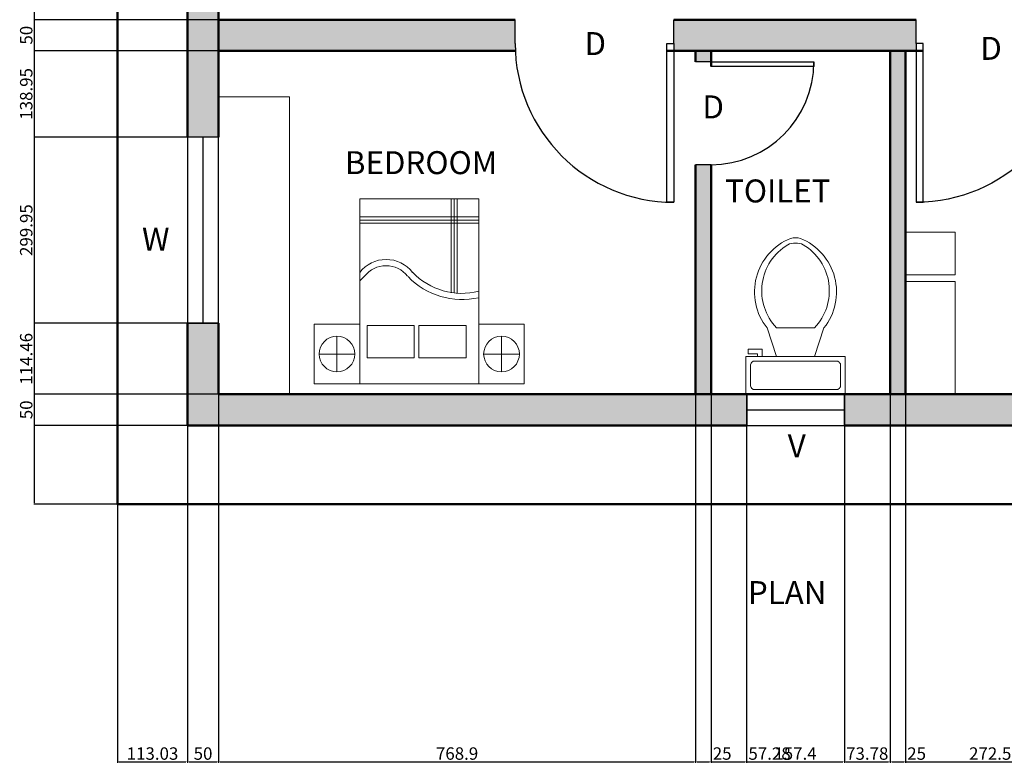
# Model space of a CAD drawing. Units: millimetres. Extents: x 1898 to 8115, y 727 to 4291.
# Tile 3 of 7: x 5191 to 6778, y 1079 to 2277. Entities that reach past the tile are written whole.
import ezdxf

# ---------------------------------------------------------------- set-up
doc = ezdxf.new("R2010")
doc.units = ezdxf.units.MM
for name, color, linetype, lineweight in [('A-ANNO-DIMS', 2, 'Continuous', 18), ('A-ANNO-TEXT', 7, 'Continuous', 25), ('A-AREA-IDEN', 3, 'Continuous', 25), ('A-DOOR', 3, 'Continuous', 25), ('A-FLOR-FIXT', 9, 'Continuous', 18), ('A-FURN', 8, 'Continuous', 18), ('A-GLAZ', 4, 'Continuous', 25), ('A-WALL', 7, 'Continuous', 50), ('A-WALL-PATT', 8, 'Continuous', 13)]:
    doc.layers.add(name, color=color, linetype=linetype, lineweight=lineweight)
doc.styles.get("Standard").update_dxf_attribs({"font": 'arial.ttf'})
doc.dimstyles.new('ISO-25', dxfattribs={"dimtxt": 20, "dimasz": 2.5, "dimexe": 1.25, "dimexo": 0.625, "dimtad": 1, "dimtxsty": 'Standard', "dimcen": 2.5, "dimadec": 0, "dimazin": 0, "dimtfac": 1, "dimtmove": 0, "dimatfit": 3, "dimfxl": 1, "dimarcsym": 0})

# ---------------------------------------------------------------- blocks, each defined once
blk = doc.blocks.new('*U43')
for p, q in [((0, 0), (0, -6)), ((40, 0), (40, -6))]:
    blk.add_line(p, q)
blk.add_lwpolyline([(0, 0), (0, 40), (1.75, 40), (1.75, 0)], close=True)
blk.add_arc((0, 0), 40, 0, 90)
blk = doc.blocks.new('*U45')
for p, q in [((9.5, -6), (9.5, -2)), ((-8, -8.5), (-8, -8)), ((-7, -8), (-7, -9.5)), ((-4, -8), (-6, -14)), ((4, -8), (6, -14)), ((-10, -8.5), (-8, -8.5)), ((-10, -9.5), (-10, -8.5)), ((-7, -9.5), (-10, -9.5)), ((4, -14), (-4, -14))]:
    blk.add_line(p, q)
blk.add_lwpolyline([(10.5, -8), (10.5, 0), (-10.5, 0), (-10.5, -8)], close=True)
for points in [[(-9.5, -2), (-9.5, -6)], [(8.5, -1), (-8.5, -1)], [(-8.5, -7), (8.5, -7)]]:
    blk.add_lwpolyline(points)
for centre, radius, start, end in [((-8.62, -1.88), 0.884, 81.8699, 188.1301), ((8.62, -1.88), 0.884, 351.8699, 98.1301), ((-8.62, -6.12), 0.884, 171.8699, 278.1301), ((8.62, -6.12), 0.884, 261.8699, 8.1301), ((3.52, -21.58), 12.17, 141.4691, 247.9714), ((4.2, -21.82), 11.33, 136.3677, 238.9468), ((-3.52, -21.58), 12.17, 292.0284, 38.5307), ((-4.2, -21.82), 11.33, 301.053, 43.6321), ((0, -27.88), 4, 245.7318, 294.2682), ((0, -29), 4, 254.8605, 285.1395)]:
    blk.add_arc(centre, radius, start, end)
blk = doc.blocks.new('BED-DOUBLE-SET')
for p, q in [((5578.8, 3262.9), (5578.8, 3320.5)), ((5550, 3291.7), (5607.6, 3291.7)), ((5704.8, 3246.7), (5696.6, 3255)), ((5789.5, 3063.1), (5789.5, 3255)), ((5794.5, 3063.1), (5794.5, 3255)), ((5799.5, 3063.1), (5799.5, 3255)), ((5677.2, 3107.9), (5828.6, 3107.9)), ((5677.2, 3102.9), (5828.6, 3102.9)), ((5677.2, 3097.9), (5828.6, 3097.9)), ((5578.8, 2997.7), (5578.8, 3055.3)), ((5550, 3026.5), (5607.6, 3026.5))]:
    blk.add_line(p, q)
for points in [[(5530.8, 3255), (5626.9, 3255), (5626.9, 3328.4), (5530.8, 3328.4)], [(5530.8, 3255), (5828.6, 3255), (5828.6, 3063.1), (5530.8, 3063.1)], [(5572.7, 3167.2), (5624.7, 3167.2), (5624.7, 3243.2), (5572.7, 3243.2)], [(5572.7, 3083.7), (5624.7, 3083.7), (5624.7, 3159.7), (5572.7, 3159.7)], [(5530.8, 2989.8), (5626.9, 2989.8), (5626.9, 3063.1), (5530.8, 3063.1)]]:
    blk.add_lwpolyline(points, close=True)
for centre in [(5578.8, 3291.7), (5578.8, 3026.5)]:
    blk.add_circle(centre, 28.8)
for centre, radius, start, end in [((5677.1, 3212.5), 54, 307.9745, 52.0255), ((5677.1, 3212.5), 44, 307.9745, 52.0255), ((5787.6, 3090), 121.1, 134.0052, 192.8109), ((5787.6, 3090), 111.1, 134.0052, 193.986)]:
    blk.add_arc(centre, radius, start, end)
blk = doc.blocks.new('*D59')
at = {"layer": 'A-ANNO-DIMS', "color": 0, "lineweight": -2, "transparency": 16777216}
for p, q in [((5347.9, 3559.7), (5213.8, 3559.7)), ((5215.1, 1499), (5215.1, 3557.2)), ((5347.9, 1496.5), (5213.8, 1496.5))]:
    blk.add_line(p, q, dxfattribs=at)
at = {"layer": 'A-ANNO-DIMS', "color": 0, "transparency": 16777216}
for points in [[(5214.6, 3557.2), (5215.5, 3557.2), (5215.1, 3559.7)], [(5214.6, 1499), (5215.5, 1499), (5215.1, 1496.5)]]:
    blk.add_solid(points, dxfattribs=at)
at = {"layer": 'Defpoints', "color": 0, "transparency": 16777216}
for p in [(5215.1, 3559.7), (5348.6, 3559.7), (5348.6, 1496.5)]:
    blk.add_point(p, dxfattribs=at)
at = {"layer": 'A-ANNO-DIMS', "color": 0, "transparency": 16777216, "insert": (5204.2, 2528.1), "char_height": 20, "attachment_point": 5, "rotation": 90}
blk.add_mtext('2063', dxfattribs=at)
blk = doc.blocks.new('*D60')
at = {"layer": 'A-ANNO-DIMS', "color": 0, "lineweight": -2, "transparency": 16777216}
for p, q in [((5461, 3440.7), (5213.8, 3440.7)), ((5215.1, 1626.1), (5215.1, 3438.2)), ((5461, 1623.6), (5213.8, 1623.6))]:
    blk.add_line(p, q, dxfattribs=at)
at = {"layer": 'A-ANNO-DIMS', "color": 0, "transparency": 16777216}
for points in [[(5214.6, 3438.2), (5215.5, 3438.2), (5215.1, 3440.7)], [(5214.6, 1626.1), (5215.5, 1626.1), (5215.1, 1623.6)]]:
    blk.add_solid(points, dxfattribs=at)
at = {"layer": 'Defpoints', "color": 0, "transparency": 16777216}
for p in [(5215.1, 3440.7), (5461.6, 3440.7), (5461.6, 1623.6)]:
    blk.add_point(p, dxfattribs=at)
at = {"layer": 'A-ANNO-DIMS', "color": 0, "transparency": 16777216, "insert": (5204.2, 2532.1), "char_height": 20, "attachment_point": 5, "rotation": 90}
blk.add_mtext('1817', dxfattribs=at)
blk = doc.blocks.new('*D61')
at = {"layer": 'A-ANNO-DIMS', "color": 0, "lineweight": -2, "transparency": 16777216}
for p, q in [((5461.6, 1623), (5461.6, 1080.3)), ((5348.6, 1495.9), (5348.6, 1080.3)), ((5351.1, 1081.6), (5459.1, 1081.6))]:
    blk.add_line(p, q, dxfattribs=at)
at = {"layer": 'A-ANNO-DIMS', "color": 0, "transparency": 16777216}
for points in [[(5351.1, 1082), (5351.1, 1081.2), (5348.6, 1081.6)], [(5459.1, 1082), (5459.1, 1081.2), (5461.6, 1081.6)]]:
    blk.add_solid(points, dxfattribs=at)
at = {"layer": 'Defpoints', "color": 0, "transparency": 16777216}
for p in [(5461.6, 1623.6), (5348.6, 1496.5), (5461.6, 1081.6)]:
    blk.add_point(p, dxfattribs=at)
at = {"layer": 'A-ANNO-DIMS', "color": 0, "transparency": 16777216, "insert": (5405.1, 1092.4), "char_height": 20, "attachment_point": 5}
blk.add_mtext('113.03', dxfattribs=at)
blk = doc.blocks.new('*D70')
at = {"layer": 'A-ANNO-DIMS', "color": 0, "lineweight": -2, "transparency": 16777216}
for p, q in [((5511.6, 1673), (5511.6, 1080.3)), ((5461.6, 1623), (5461.6, 1080.3)), ((5464.1, 1081.6), (5509.1, 1081.6))]:
    blk.add_line(p, q, dxfattribs=at)
at = {"layer": 'A-ANNO-DIMS', "color": 0, "transparency": 16777216}
for points in [[(5464.1, 1082), (5464.1, 1081.2), (5461.6, 1081.6)], [(5509.1, 1082), (5509.1, 1081.2), (5511.6, 1081.6)]]:
    blk.add_solid(points, dxfattribs=at)
at = {"layer": 'Defpoints', "color": 0, "transparency": 16777216}
for p in [(5511.6, 1673.6), (5461.6, 1623.6), (5511.6, 1081.6)]:
    blk.add_point(p, dxfattribs=at)
at = {"layer": 'A-ANNO-DIMS', "color": 0, "transparency": 16777216, "insert": (5486.6, 1092.4), "char_height": 20, "attachment_point": 5}
blk.add_mtext('50', dxfattribs=at)
blk = doc.blocks.new('*D71')
at = {"layer": 'A-ANNO-DIMS', "color": 0, "lineweight": -2, "transparency": 16777216}
for p, q in [((5511.6, 1673), (5511.6, 1080.3)), ((6280.5, 1673), (6280.5, 1080.3)), ((5514.1, 1081.6), (6278, 1081.6))]:
    blk.add_line(p, q, dxfattribs=at)
at = {"layer": 'A-ANNO-DIMS', "color": 0, "transparency": 16777216}
for points in [[(5514.1, 1082), (5514.1, 1081.2), (5511.6, 1081.6)], [(6278, 1082), (6278, 1081.2), (6280.5, 1081.6)]]:
    blk.add_solid(points, dxfattribs=at)
at = {"layer": 'Defpoints', "color": 0, "transparency": 16777216}
for p in [(5511.6, 1673.6), (6280.5, 1673.6), (6280.5, 1081.6)]:
    blk.add_point(p, dxfattribs=at)
at = {"layer": 'A-ANNO-DIMS', "color": 0, "transparency": 16777216, "insert": (5896, 1092.4), "char_height": 20, "attachment_point": 5}
blk.add_mtext('768.9', dxfattribs=at)
blk = doc.blocks.new('*D72')
at = {"layer": 'A-ANNO-DIMS', "color": 0, "lineweight": -2, "transparency": 16777216}
for p, q in [((6280.5, 1673), (6280.5, 1080.3)), ((6305.5, 1673), (6305.5, 1080.3)), ((6283, 1081.6), (6303, 1081.6)), ((6305.5, 1081.6), (6338.4, 1081.6))]:
    blk.add_line(p, q, dxfattribs=at)
at = {"layer": 'A-ANNO-DIMS', "color": 0, "transparency": 16777216}
for points in [[(6283, 1082), (6283, 1081.2), (6280.5, 1081.6)], [(6303, 1082), (6303, 1081.2), (6305.5, 1081.6)]]:
    blk.add_solid(points, dxfattribs=at)
at = {"layer": 'Defpoints', "color": 0, "transparency": 16777216}
for p in [(6280.5, 1673.6), (6305.5, 1673.6), (6305.5, 1081.6)]:
    blk.add_point(p, dxfattribs=at)
at = {"layer": 'A-ANNO-DIMS', "color": 0, "transparency": 16777216, "insert": (6323.2, 1092.4), "char_height": 20, "attachment_point": 5}
blk.add_mtext('25', dxfattribs=at)
blk = doc.blocks.new('*D73')
at = {"layer": 'A-ANNO-DIMS', "color": 0, "lineweight": -2, "transparency": 16777216}
for p, q in [((6305.5, 1673), (6305.5, 1080.3)), ((6362.7, 1673), (6362.7, 1080.3)), ((6308, 1081.6), (6360.2, 1081.6)), ((6362.7, 1081.6), (6434, 1081.6))]:
    blk.add_line(p, q, dxfattribs=at)
at = {"layer": 'A-ANNO-DIMS', "color": 0, "transparency": 16777216}
for points in [[(6308, 1082), (6308, 1081.2), (6305.5, 1081.6)], [(6360.2, 1082), (6360.2, 1081.2), (6362.7, 1081.6)]]:
    blk.add_solid(points, dxfattribs=at)
at = {"layer": 'Defpoints', "color": 0, "transparency": 16777216}
for p in [(6305.5, 1673.6), (6362.7, 1673.6), (6362.7, 1081.6)]:
    blk.add_point(p, dxfattribs=at)
at = {"layer": 'A-ANNO-DIMS', "color": 0, "transparency": 16777216, "insert": (6399.6, 1092.4), "char_height": 20, "attachment_point": 5}
blk.add_mtext('57.28', dxfattribs=at)
blk = doc.blocks.new('*D74')
at = {"layer": 'A-ANNO-DIMS', "color": 0, "lineweight": -2, "transparency": 16777216}
for p, q in [((6362.7, 1673), (6362.7, 1080.3)), ((6520.2, 1673), (6520.2, 1080.3)), ((6365.2, 1081.6), (6517.7, 1081.6))]:
    blk.add_line(p, q, dxfattribs=at)
at = {"layer": 'A-ANNO-DIMS', "color": 0, "transparency": 16777216}
for points in [[(6365.2, 1082), (6365.2, 1081.2), (6362.7, 1081.6)], [(6517.7, 1082), (6517.7, 1081.2), (6520.2, 1081.6)]]:
    blk.add_solid(points, dxfattribs=at)
at = {"layer": 'Defpoints', "color": 0, "transparency": 16777216}
for p in [(6362.7, 1673.6), (6520.2, 1673.6), (6520.2, 1081.6)]:
    blk.add_point(p, dxfattribs=at)
at = {"layer": 'A-ANNO-DIMS', "color": 0, "transparency": 16777216, "insert": (6441.4, 1092.4), "char_height": 20, "attachment_point": 5}
blk.add_mtext('157.4', dxfattribs=at)
blk = doc.blocks.new('*D75')
at = {"layer": 'A-ANNO-DIMS', "color": 0, "lineweight": -2, "transparency": 16777216}
for p, q in [((6520.2, 1673), (6520.2, 1080.3)), ((6593.9, 1673), (6593.9, 1080.3)), ((6522.7, 1081.6), (6591.4, 1081.6))]:
    blk.add_line(p, q, dxfattribs=at)
at = {"layer": 'A-ANNO-DIMS', "color": 0, "transparency": 16777216}
for points in [[(6522.7, 1082), (6522.7, 1081.2), (6520.2, 1081.6)], [(6591.4, 1082), (6591.4, 1081.2), (6593.9, 1081.6)]]:
    blk.add_solid(points, dxfattribs=at)
at = {"layer": 'Defpoints', "color": 0, "transparency": 16777216}
for p in [(6520.2, 1673.6), (6593.9, 1673.6), (6593.9, 1081.6)]:
    blk.add_point(p, dxfattribs=at)
at = {"layer": 'A-ANNO-DIMS', "color": 0, "transparency": 16777216, "insert": (6557, 1092.4), "char_height": 20, "attachment_point": 5}
blk.add_mtext('73.78', dxfattribs=at)
blk = doc.blocks.new('*D76')
at = {"layer": 'A-ANNO-DIMS', "color": 0, "lineweight": -2, "transparency": 16777216}
for p, q in [((6593.9, 1673), (6593.9, 1080.3)), ((6618.9, 1673), (6618.9, 1080.3)), ((6596.4, 1081.6), (6616.4, 1081.6)), ((6618.9, 1081.6), (6651.8, 1081.6))]:
    blk.add_line(p, q, dxfattribs=at)
at = {"layer": 'A-ANNO-DIMS', "color": 0, "transparency": 16777216}
for points in [[(6596.4, 1082), (6596.4, 1081.2), (6593.9, 1081.6)], [(6616.4, 1082), (6616.4, 1081.2), (6618.9, 1081.6)]]:
    blk.add_solid(points, dxfattribs=at)
at = {"layer": 'Defpoints', "color": 0, "transparency": 16777216}
for p in [(6593.9, 1673.6), (6618.9, 1673.6), (6618.9, 1081.6)]:
    blk.add_point(p, dxfattribs=at)
at = {"layer": 'A-ANNO-DIMS', "color": 0, "transparency": 16777216, "insert": (6636.6, 1092.4), "char_height": 20, "attachment_point": 5}
blk.add_mtext('25', dxfattribs=at)
blk = doc.blocks.new('*D77')
at = {"layer": 'A-ANNO-DIMS', "color": 0, "lineweight": -2, "transparency": 16777216}
for p, q in [((6618.9, 1673), (6618.9, 1080.3)), ((7265.8, 1673), (7265.8, 1080.3)), ((6621.4, 1081.6), (7263.3, 1081.6))]:
    blk.add_line(p, q, dxfattribs=at)
at = {"layer": 'A-ANNO-DIMS', "color": 0, "transparency": 16777216}
for points in [[(6621.4, 1082), (6621.4, 1081.2), (6618.9, 1081.6)], [(7263.3, 1082), (7263.3, 1081.2), (7265.8, 1081.6)]]:
    blk.add_solid(points, dxfattribs=at)
at = {"layer": 'Defpoints', "color": 0, "transparency": 16777216}
for p in [(6618.9, 1673.6), (7265.8, 1673.6), (7265.8, 1081.6)]:
    blk.add_point(p, dxfattribs=at)
at = {"layer": 'A-ANNO-DIMS', "color": 0, "transparency": 16777216, "insert": (6942.3, 1092.4), "char_height": 20, "attachment_point": 5}
blk.add_mtext('646.8', dxfattribs=at)
blk = doc.blocks.new('*D79')
at = {"layer": 'A-ANNO-DIMS', "color": 0, "lineweight": -2, "transparency": 16777216}
for p, q in [((5511, 1673.6), (5213.8, 1673.6)), ((5215.1, 1626.1), (5215.1, 1671.1)), ((5461, 1623.6), (5213.8, 1623.6))]:
    blk.add_line(p, q, dxfattribs=at)
at = {"layer": 'A-ANNO-DIMS', "color": 0, "transparency": 16777216}
for points in [[(5214.6, 1671.1), (5215.5, 1671.1), (5215.1, 1673.6)], [(5214.6, 1626.1), (5215.5, 1626.1), (5215.1, 1623.6)]]:
    blk.add_solid(points, dxfattribs=at)
at = {"layer": 'Defpoints', "color": 0, "transparency": 16777216}
for p in [(5215.1, 1673.6), (5511.6, 1673.6), (5461.6, 1623.6)]:
    blk.add_point(p, dxfattribs=at)
at = {"layer": 'A-ANNO-DIMS', "color": 0, "transparency": 16777216, "insert": (5204.2, 1648.6), "char_height": 20, "attachment_point": 5, "rotation": 90}
blk.add_mtext('50', dxfattribs=at)
blk = doc.blocks.new('*D80')
at = {"layer": 'A-ANNO-DIMS', "color": 0, "lineweight": -2, "transparency": 16777216}
for p, q in [((5511, 1788.1), (5213.8, 1788.1)), ((5215.1, 1676.1), (5215.1, 1785.6)), ((5511, 1673.6), (5213.8, 1673.6))]:
    blk.add_line(p, q, dxfattribs=at)
at = {"layer": 'A-ANNO-DIMS', "color": 0, "transparency": 16777216}
for points in [[(5214.6, 1785.6), (5215.5, 1785.6), (5215.1, 1788.1)], [(5214.6, 1676.1), (5215.5, 1676.1), (5215.1, 1673.6)]]:
    blk.add_solid(points, dxfattribs=at)
at = {"layer": 'Defpoints', "color": 0, "transparency": 16777216}
for p in [(5215.1, 1788.1), (5511.6, 1788.1), (5511.6, 1673.6)]:
    blk.add_point(p, dxfattribs=at)
at = {"layer": 'A-ANNO-DIMS', "color": 0, "transparency": 16777216, "insert": (5204.2, 1730.8), "char_height": 20, "attachment_point": 5, "rotation": 90}
blk.add_mtext('114.46', dxfattribs=at)
blk = doc.blocks.new('*D81')
at = {"layer": 'A-ANNO-DIMS', "color": 0, "lineweight": -2, "transparency": 16777216}
for p, q in [((5511, 2088), (5213.8, 2088)), ((5215.1, 1790.6), (5215.1, 2085.5)), ((5511, 1788.1), (5213.8, 1788.1))]:
    blk.add_line(p, q, dxfattribs=at)
at = {"layer": 'A-ANNO-DIMS', "color": 0, "transparency": 16777216}
for points in [[(5214.6, 2085.5), (5215.5, 2085.5), (5215.1, 2088)], [(5214.6, 1790.6), (5215.5, 1790.6), (5215.1, 1788.1)]]:
    blk.add_solid(points, dxfattribs=at)
at = {"layer": 'Defpoints', "color": 0, "transparency": 16777216}
for p in [(5215.1, 2088), (5511.6, 2088), (5511.6, 1788.1)]:
    blk.add_point(p, dxfattribs=at)
at = {"layer": 'A-ANNO-DIMS', "color": 0, "transparency": 16777216, "insert": (5204.2, 1938.1), "char_height": 20, "attachment_point": 5, "rotation": 90}
blk.add_mtext('299.95', dxfattribs=at)
blk = doc.blocks.new('*D82')
at = {"layer": 'A-ANNO-DIMS', "color": 0, "lineweight": -2, "transparency": 16777216}
for p, q in [((5511, 2227), (5213.8, 2227)), ((5215.1, 2090.5), (5215.1, 2224.5)), ((5511, 2088), (5213.8, 2088))]:
    blk.add_line(p, q, dxfattribs=at)
at = {"layer": 'A-ANNO-DIMS', "color": 0, "transparency": 16777216}
for points in [[(5214.6, 2224.5), (5215.5, 2224.5), (5215.1, 2227)], [(5214.6, 2090.5), (5215.5, 2090.5), (5215.1, 2088)]]:
    blk.add_solid(points, dxfattribs=at)
at = {"layer": 'Defpoints', "color": 0, "transparency": 16777216}
for p in [(5215.1, 2227), (5511.6, 2227), (5511.6, 2088)]:
    blk.add_point(p, dxfattribs=at)
at = {"layer": 'A-ANNO-DIMS', "color": 0, "transparency": 16777216, "insert": (5204.2, 2157.5), "char_height": 20, "attachment_point": 5, "rotation": 90}
blk.add_mtext('138.95', dxfattribs=at)
blk = doc.blocks.new('*D83')
at = {"layer": 'A-ANNO-DIMS', "color": 0, "lineweight": -2, "transparency": 16777216}
for p, q in [((5511, 2277), (5213.8, 2277)), ((5215.1, 2229.5), (5215.1, 2274.5)), ((5511, 2227), (5213.8, 2227))]:
    blk.add_line(p, q, dxfattribs=at)
at = {"layer": 'A-ANNO-DIMS', "color": 0, "transparency": 16777216}
for points in [[(5214.6, 2274.5), (5215.5, 2274.5), (5215.1, 2277)], [(5214.6, 2229.5), (5215.5, 2229.5), (5215.1, 2227)]]:
    blk.add_solid(points, dxfattribs=at)
at = {"layer": 'Defpoints', "color": 0, "transparency": 16777216}
for p in [(5215.1, 2277), (5511.6, 2277), (5511.6, 2227)]:
    blk.add_point(p, dxfattribs=at)
at = {"layer": 'A-ANNO-DIMS', "color": 0, "transparency": 16777216, "insert": (5204.2, 2252), "char_height": 20, "attachment_point": 5, "rotation": 90}
blk.add_mtext('50', dxfattribs=at)
blk = doc.blocks.new('*D107')
at = {"layer": 'A-ANNO-DIMS', "color": 0, "lineweight": -2, "transparency": 16777216}
for p, q in [((6618.9, 2226.3), (6618.9, 1080.3)), ((6891.4, 2226.3), (6891.4, 1080.3)), ((6621.4, 1081.6), (6888.9, 1081.6))]:
    blk.add_line(p, q, dxfattribs=at)
at = {"layer": 'A-ANNO-DIMS', "color": 0, "transparency": 16777216}
for points in [[(6621.4, 1082), (6621.4, 1081.2), (6618.9, 1081.6)], [(6888.9, 1082), (6888.9, 1081.2), (6891.4, 1081.6)]]:
    blk.add_solid(points, dxfattribs=at)
at = {"layer": 'Defpoints', "color": 0, "transparency": 16777216}
for p in [(6618.9, 2227), (6891.4, 2227), (6891.4, 1081.6)]:
    blk.add_point(p, dxfattribs=at)
at = {"layer": 'A-ANNO-DIMS', "color": 0, "transparency": 16777216, "insert": (6755.2, 1092.4), "char_height": 20, "attachment_point": 5}
blk.add_mtext('272.5', dxfattribs=at)

msp = doc.modelspace()

# ---------------------------------------------------------------- hatches: boundary and pattern name
at = {"layer": 'A-WALL-PATT'}
h = msp.add_hatch(color=256, dxfattribs=at)
h.dxf.hatch_style = 1
h.paths.add_polyline_path([(6201.726, 3440.661), (5461.585, 3440.661), (5461.585, 3265.221), (5511.585, 3265.221), (5511.585, 3390.661), (6176.726, 3390.661), (6176.726, 2856.284), (6201.726, 2856.284)])
h.paths.add_polyline_path([(6784.895, 3318.017), (6201.726, 3318.017), (6201.726, 3268.017), (6784.895, 3268.017)])
h.paths.add_polyline_path([(7570.217, 3440.661), (6784.895, 3440.661), (6784.895, 3057.009), (6809.895, 3057.009), (6809.895, 3390.661), (7520.217, 3390.661), (7520.217, 3300.311), (7570.217, 3300.311)])
h.paths.add_polyline_path([(7570.217, 3000.359), (7520.217, 3000.359), (7520.217, 2758.681), (7570.217, 2758.681)])
h.paths.add_polyline_path([(7520.217, 2856.284), (7194.283, 2856.284), (6784.895, 2856.284), (6784.895, 2831.284), (7520.217, 2831.284)])
h.paths.add_polyline_path([(6809.895, 2878.069), (6784.895, 2878.069), (6784.895, 2856.284), (6809.895, 2856.284)])
h.paths.add_polyline_path([(6201.726, 2856.284), (6176.726, 2856.284), (6161.551, 2856.284), (6161.551, 2831.284), (6201.726, 2831.284)])
h.paths.add_polyline_path([(5905.861, 2856.284), (5511.585, 2856.284), (5511.585, 2831.284), (5905.861, 2831.284)])
h.paths.add_polyline_path([(5511.585, 2965.269), (5461.585, 2965.269), (5461.585, 2698.678), (5511.585, 2698.678)])
h.paths.add_polyline_path([(5511.585, 2398.725), (5461.585, 2398.725), (5461.585, 2088.028), (5511.585, 2088.028)])
h.paths.add_polyline_path([(5989.6, 2238.621), (5989.6, 2276.975), (5511.585, 2276.975), (5511.585, 2226.975), (5989.865, 2226.975, -0.01139164)])
h.paths.add_polyline_path([(6636.013, 2276.975), (6245.29, 2276.975), (6245.29, 2238.621), (6245.29, 2226.975), (6636.013, 2226.975), (6636.013, 2238.621)])
h.paths.add_polyline_path([(7570.217, 2359.481), (7520.217, 2359.481), (7520.217, 2326.802), (7520.217, 2276.975), (6891.704, 2276.975), (6891.704, 2238.621, -0.01139164), (6891.439, 2226.975), (7570.217, 2226.975)])
h.paths.add_polyline_path([(7145.586, 2531.644), (6989.313, 2531.644), (6989.313, 2538.488), (7145.735, 2538.488), (7145.735, 2531.644), (7145.586, 2531.644, -0.39860379), (6990.849, 2382.073), (6990.849, 2276.975), (6965.849, 2276.975), (6965.849, 2382.065), (6989.313, 2382.065, 0.40145271)])
h.paths.add_polyline_path([(6990.849, 2596.561), (6989.313, 2596.561), (6965.849, 2596.561), (6965.849, 2538.488), (6990.849, 2538.488)])
h.paths.add_polyline_path([(6990.849, 2831.284), (6965.849, 2831.284), (6965.849, 2752.984), (6990.849, 2752.984)])
h.paths.add_polyline_path([(7570.217, 2638.517), (7520.217, 2638.517), (7520.217, 2625.002), (7520.217, 2479.644), (7570.217, 2479.644)])
h.paths.add_polyline_path([(7520.217, 2579.13), (6990.849, 2579.13), (6990.849, 2554.13), (7520.217, 2554.13)])
h = msp.add_hatch(color=256, dxfattribs=at)
h.dxf.hatch_style = 1
h.paths.add_polyline_path([(6362.741, 1673.621), (6361.204, 1673.621), (5511.585, 1673.621), (5511.585, 1788.076), (5461.585, 1788.076), (5461.585, 1623.621), (6362.741, 1623.621)])
h.paths.add_polyline_path([(7315.762, 1755.132), (7265.762, 1755.132), (7265.762, 1673.621), (6520.151, 1673.621), (6520.151, 1623.621), (7315.762, 1623.621)])
h.paths.add_polyline_path([(7315.762, 2226.975), (7265.762, 2226.975), (7265.762, 2168.705), (7265.762, 2055.084), (7315.762, 2055.084)])
h.paths.add_polyline_path([(6618.931, 1855.35), (6618.931, 2226.975), (6593.931, 2226.975), (6593.931, 1673.621), (6618.931, 1673.621)])
h.paths.add_polyline_path([(6305.461, 2043.361), (6280.461, 2043.361), (6280.461, 1673.621), (6305.461, 1673.621)])
h.paths.add_polyline_path([(6305.461, 2226.975), (6280.461, 2226.975), (6280.461, 2209.076), (6305.461, 2209.076)])

# ---------------------------------------------------------------- linework, layer by layer
at = {"layer": 'A-FURN'}
msp.add_lwpolyline([(5511.585, 1788.076), (5511.585, 1673.621), (5626.005, 1673.621), (5626.005, 2152.55), (5511.585, 2152.55), (5511.585, 2088.028)], dxfattribs=at)
for points in [[(6618.931, 1866.197), (6698.95, 1866.197), (6698.95, 1934.623), (6618.931, 1934.623)], [(6618.931, 1673.621), (6698.836, 1673.621), (6698.836, 1855.35), (6618.931, 1855.35)]]:
    msp.add_lwpolyline(points, close=True, dxfattribs=at)
at = {"layer": 'A-GLAZ'}
for p, q in [((5486.585, 1788.076), (5486.585, 2088.028)), ((6362.741, 1648.621), (6520.151, 1648.621))]:
    msp.add_line(p, q, dxfattribs=at)
for points in [[(5511.585, 2088.028), (5461.585, 2088.028)], [(5461.585, 1788.076), (5511.585, 1788.076)], [(6362.741, 1623.621), (6362.741, 1673.621), (6520.151, 1673.621), (6520.151, 1623.621)]]:
    msp.add_lwpolyline(points, dxfattribs=at)
for points in [[(5461.585, 1788.076), (5511.585, 1788.076), (5511.585, 2088.028), (5461.585, 2088.028)], [(6362.741, 1623.621), (6520.151, 1623.621), (6520.151, 1673.621), (6362.741, 1673.621)]]:
    msp.add_lwpolyline(points, close=True, dxfattribs=at)
at = {"layer": 'A-WALL'}
for p, q in [((5461.585, 2088.028), (5461.585, 2398.725)), ((5511.585, 2088.028), (5511.585, 2398.725)), ((5511.585, 2276.975), (5989.6, 2276.975)), ((6245.29, 2276.975), (6636.013, 2276.975)), ((5511.585, 2226.975), (5989.865, 2226.975)), ((6234.104, 2226.975), (6647.2, 2226.975)), ((6280.461, 2226.975), (6280.461, 2209.076)), ((6305.461, 2226.975), (6305.461, 2201.826)), ((6593.931, 2226.975), (6593.931, 1673.621)), ((6618.931, 2226.975), (6618.931, 1673.621)), ((6280.461, 2043.361), (6280.461, 1673.621)), ((6305.461, 2043.361), (6305.461, 1673.621)), ((5461.585, 1623.621), (5461.585, 1788.076)), ((5511.585, 1673.621), (5511.585, 1788.076)), ((5511.585, 1673.621), (7265.762, 1673.621)), ((5461.585, 1623.621), (6362.741, 1623.621)), ((6520.151, 1623.621), (7315.762, 1623.621))]:
    msp.add_line(p, q, dxfattribs=at)
msp.add_lwpolyline([(5348.551, 3559.737), (7698.767, 3559.737), (7698.767, 1496.544), (5348.551, 1496.544)], close=True, dxfattribs=at)

# ---------------------------------------------------------------- block references
at = {"layer": 'A-DOOR'}
for p, xscale, yscale, zscale, rotation in [((6245.29, 2238.621), 6.392265120440044, 6.392265120440044, 6.392265120440044, 180), ((6636.013, 2238.621), -6.392265120440044, 6.392265120440044, 6.392265120440044, 180), ((6305.318, 2209.076), 4.142879620656954, 4.142879620656954, 4.142879620656954, 270)]:
    msp.add_blockref('*U43', p, dxfattribs=dict(at, xscale=xscale, yscale=yscale, zscale=zscale, rotation=rotation))
at = {"layer": 'A-FLOR-FIXT', "xscale": -7.642125996577618, "yscale": 7.642125996577618, "zscale": 7.642125996577618, "rotation": 180}
msp.add_blockref('*U45', (6441.446, 1673.621), dxfattribs=at)
at = {"layer": 'A-FURN', "rotation": 90.00000000000011}
msp.add_blockref('BED-DOUBLE-SET', (8994.138, -3840.286), dxfattribs=at)

# ---------------------------------------------------------------- texts
at = {"layer": 'A-ANNO-TEXT', "attachment_point": 1}
for s, insert, char_height in [('D', (6101.335, 2257.036), 36.981), ('D', (6739.231, 2249.317), 36.981), ('D', (6291.443, 2155.047), 36.981), ('W', (5388.184, 1942.069), 36.981), ('V', (6428.916, 1608.966), 36.981), ('PLAN', (6364.74, 1372.714), 36.9814)]:
    msp.add_mtext_dynamic_manual_height_columns(s, width=5503.90807, gutter_width=184.907, heights=[0], dxfattribs=dict(at, insert=insert, char_height=char_height))
at = {"layer": 'A-AREA-IDEN', "char_height": 36.9814, "attachment_point": 1}
for s, insert in [('BEDROOM', (5715.198, 2065.234)), ('TOILET', (6327.932, 2019.621))]:
    msp.add_mtext_dynamic_manual_height_columns(s, width=5503.90807, gutter_width=184.907, heights=[0], dxfattribs=dict(at, insert=insert))

# ---------------------------------------------------------------- dimensions: what is measured, and where the dimension line sits
at = {"layer": 'A-ANNO-DIMS'}
for base, p1, p2, override, picture, middle in [((5215.051, 3559.737), (5348.551, 1496.544), (5348.551, 3559.737), {"dimdec": 0, "dimlfac": 1, "dimrnd": 0, "dimzin": 0, "dimdsep": 46, "dimlunit": 2}, '*D59', (5204.207, 2528.14)), ((5215.051, 3440.661), (5461.585, 1623.621), (5461.585, 3440.661), {"dimdec": 0, "dimlfac": 1, "dimrnd": 0, "dimzin": 0, "dimdsep": 46, "dimlunit": 2}, '*D60', (5204.214, 2532.141)), ((5215.051, 2276.975), (5511.585, 2226.975), (5511.585, 2276.975), {"dimdec": 0, "dimlfac": 1, "dimrnd": 0, "dimzin": 0, "dimdsep": 46, "dimlunit": 2}, '*D83', (5204.214, 2251.975)), ((5215.051, 2226.975), (5511.585, 2088.028), (5511.585, 2226.975), {"dimdec": 2, "dimlfac": 1, "dimrnd": 0, "dimzin": 0, "dimdsep": 46, "dimlunit": 2}, '*D82', (5204.207, 2157.502)), ((5215.051, 2088.028), (5511.585, 1788.076), (5511.585, 2088.028), {"dimdec": 2, "dimlfac": 1, "dimrnd": 0, "dimzin": 0, "dimdsep": 46, "dimlunit": 2}, '*D81', (5204.214, 1938.052)), ((5215.05059, 1788.07612), (5511.58477, 1673.62111), (5511.58477, 1788.07612), {"dimdec": 2, "dimlfac": 1, "dimrnd": 0, "dimzin": 0, "dimdsep": 46, "dimlunit": 2}, '*D80', (5204.21413, 1730.84861)), ((5215.051, 1673.621), (5461.585, 1623.621), (5511.585, 1673.621), {"dimdec": 0, "dimlfac": 1, "dimrnd": 0, "dimzin": 0, "dimdsep": 46, "dimlunit": 2}, '*D79', (5204.214, 1648.621))]:
    dim = msp.add_linear_dim(base=base, p1=p1, p2=p2, angle=90, dimstyle='ISO-25', override=override, dxfattribs=at)
    dim.commit()
    dim.dimension.update_dxf_attribs({"geometry": picture, "text_midpoint": middle})
for base, p1, p2, override, picture, middle in [((6891.439, 1081.594), (6618.931, 2226.975), (6891.439, 2226.975), {"dimdec": 1, "dimlfac": 1, "dimrnd": 0, "dimzin": 0, "dimdsep": 46, "dimlunit": 2}, '*D107', (6755.185, 1092.43)), ((5511.585, 1081.594), (5461.585, 1623.621), (5511.585, 1673.621), {"dimdec": 0, "dimlfac": 1, "dimrnd": 0, "dimzin": 0, "dimdsep": 46, "dimlunit": 2}, '*D70', (5486.585, 1092.43)), ((6280.461, 1081.594), (5511.585, 1673.621), (6280.461, 1673.621), {"dimdec": 1, "dimlfac": 1, "dimrnd": 0, "dimzin": 0, "dimdsep": 46, "dimlunit": 2}, '*D71', (5896.023, 1092.43)), ((6305.461, 1081.594), (6280.461, 1673.621), (6305.461, 1673.621), {"dimdec": 0, "dimlfac": 1, "dimrnd": 0, "dimzin": 0, "dimdsep": 46, "dimlunit": 2}, '*D72', (6323.156, 1092.43)), ((6362.741, 1081.594), (6305.461, 1673.621), (6362.741, 1673.621), {"dimdec": 2, "dimlfac": 1, "dimrnd": 0, "dimzin": 0, "dimdsep": 46, "dimlunit": 2}, '*D73', (6399.632, 1092.43)), ((6520.151, 1081.594), (6362.741, 1673.621), (6520.151, 1673.621), {"dimdec": 1, "dimlfac": 1, "dimrnd": 0, "dimzin": 0, "dimdsep": 46, "dimlunit": 2}, '*D74', (6441.446, 1092.43)), ((6593.931, 1081.594), (6520.151, 1673.621), (6593.931, 1673.621), {"dimdec": 2, "dimlfac": 1, "dimrnd": 0, "dimzin": 0, "dimdsep": 46, "dimlunit": 2}, '*D75', (6557.041, 1092.437)), ((6618.931, 1081.594), (6593.931, 1673.621), (6618.931, 1673.621), {"dimdec": 0, "dimlfac": 1, "dimrnd": 0, "dimzin": 0, "dimdsep": 46, "dimlunit": 2}, '*D76', (6636.626, 1092.43)), ((7265.762, 1081.594), (6618.931, 1673.621), (7265.762, 1673.621), {"dimdec": 1, "dimlfac": 1, "dimrnd": 0, "dimzin": 0, "dimdsep": 46, "dimlunit": 2}, '*D77', (6942.347, 1092.43)), ((5461.585, 1081.594), (5348.551, 1496.544), (5461.585, 1623.621), {"dimdec": 2, "dimlfac": 1, "dimrnd": 0, "dimzin": 0, "dimdsep": 46, "dimlunit": 2}, '*D61', (5405.068, 1092.437))]:
    dim = msp.add_linear_dim(base=base, p1=p1, p2=p2, dimstyle='ISO-25', override=override, dxfattribs=at)
    dim.commit()
    dim.dimension.update_dxf_attribs({"geometry": picture, "text_midpoint": middle})

doc.saveas('drawing.dxf')
